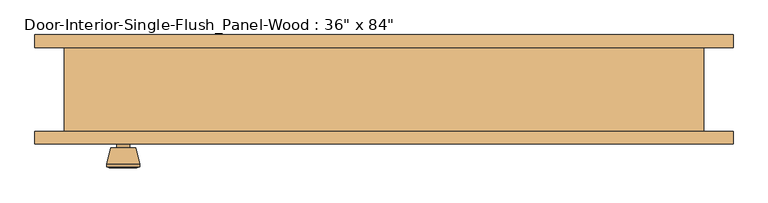
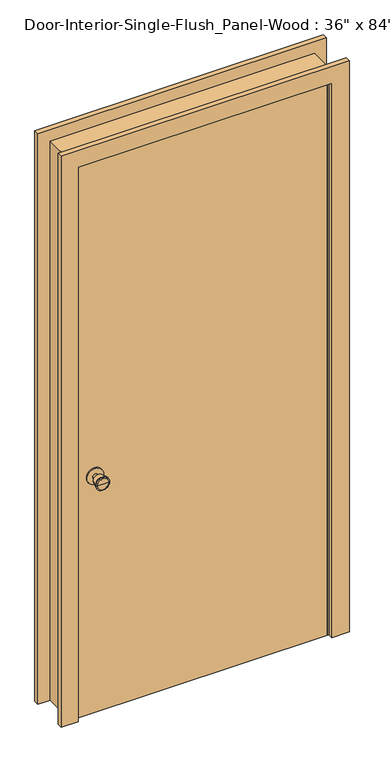
"""IFC4 building model written with IfcOpenShell, lengths in millimetres: door geometry."""

from ifc_helpers import new_model, si_unit, point, frame, frame_2d, origin, origin_with_axes, place, context, project, spatial, polyline, circle_curve, trimmed, segment, composite_curve, outline, extrude, faceted_brep, source, transform, mapped, element, save
from ifc_brep_helpers import plane_surface, cylinder_surface, revolved_surface, advanced_brep


def door_fdc9072e(model_context):
    return source(origin(), model_context, "Body", "SolidModel", [
        advanced_brep(
        [(-393.7, -19.4, 914.4), (-403.7, -19.4, 914.4), (-383.7, -19.4, 914.4), (-373.2241324, 29.6, 914.4), (-414.1758676, 29.6, 914.4), (-393.7, 29.6, 914.4), (-368.7, 27.7721319, 914.4), (-418.7, 27.7721319, 914.4), (-368.7, 24.3084537, 914.4), (-418.7, 24.3084537, 914.4), (-375.063764, -0.4, 914.4), (-412.336236, -0.4, 914.4), (-383.7, -0.4, 914.4), (-403.7, -0.4, 914.4)],
        [
            (0, 1),
            (1, 2, circle_curve(frame((-393.7, -19.4, 914.4), z_axis=(0.0, -1.0, 0.0), x_axis=(-1.0, 0.0, 0.0)), 10.0)),
            (2, 0),
            (2, 1, circle_curve(frame((-393.7, -19.4, 914.4), z_axis=(0.0, -1.0, 0.0), x_axis=(-1.0, 0.0, 0.0)), 10.0)),
            (3, 4, circle_curve(frame((-393.7, 29.6, 914.4), z_axis=(0.0, 1.0, 0.0), x_axis=(-1.0, 0.0, 0.0)), 20.4758676)),
            (4, 5),
            (5, 3),
            (4, 3, circle_curve(frame((-393.7, 29.6, 914.4), z_axis=(0.0, 1.0, 0.0), x_axis=(-1.0, 0.0, 0.0)), 20.4758676)),
            (6, 7, circle_curve(frame((-393.7, 27.7721319, 914.4), z_axis=(0.0, 1.0, 0.0), x_axis=(-1.0, 0.0, 0.0)), 25.0)),
            (7, 4),
            (3, 6),
            (7, 6, circle_curve(frame((-393.7, 27.7721319, 914.4), z_axis=(0.0, 1.0, 0.0), x_axis=(-1.0, 0.0, 0.0)), 25.0)),
            (8, 9, circle_curve(frame((-393.7, 24.3084537, 914.4), z_axis=(0.0, 1.0, 0.0), x_axis=(-1.0, 0.0, 0.0)), 25.0)),
            (9, 7),
            (6, 8),
            (9, 8, circle_curve(frame((-393.7, 24.3084537, 914.4), z_axis=(0.0, 1.0, 0.0), x_axis=(-1.0, 0.0, 0.0)), 25.0)),
            (10, 11, circle_curve(frame((-393.7, -0.4, 914.4), z_axis=(0.0, 1.0, 0.0), x_axis=(-1.0, 0.0, 0.0)), 18.636236)),
            (11, 9),
            (8, 10),
            (11, 10, circle_curve(frame((-393.7, -0.4, 914.4), z_axis=(0.0, 1.0, 0.0), x_axis=(-1.0, 0.0, 0.0)), 18.636236)),
            (12, 13, circle_curve(frame((-393.7, -0.4, 914.4), z_axis=(0.0, 1.0, 0.0), x_axis=(-1.0, 0.0, 0.0)), 10.0)),
            (13, 11),
            (10, 12),
            (13, 12, circle_curve(frame((-393.7, -0.4, 914.4), z_axis=(0.0, 1.0, 0.0), x_axis=(-1.0, 0.0, 0.0)), 10.0)),
            (1, 13),
            (12, 2),
        ],
        [
            plane_surface(frame((-393.7, -19.4, 914.4), z_axis=(0.0, -1.0, 0.0), x_axis=(-1.0, 0.0, 0.0))),
            plane_surface(frame((-393.7, 29.6, 914.4), z_axis=(0.0, 1.0, 0.0), x_axis=(-1.0, 0.0, 0.0))),
            revolved_surface(polyline([(-414.1758676, 29.6, 914.4), (-418.7, 27.7721319, 914.4)]), (-393.7, -19.4, 914.4), (0.0, -1.0, 0.0)),
            cylinder_surface(frame((-393.7, -19.4, 914.4), z_axis=(0.0, -1.0, 0.0), x_axis=(-1.0, 0.0, 0.0)), 25.0),
            revolved_surface(polyline([(-418.7, 24.3084537, 914.4), (-412.336236, -0.4, 914.4)]), (-393.7, -19.4, 914.4), (0.0, -1.0, 0.0)),
            plane_surface(frame((-393.7, -0.4, 914.4), z_axis=(0.0, -1.0, 0.0), x_axis=(-1.0, 0.0, 0.0))),
            cylinder_surface(frame((-393.7, -19.4, 914.4), z_axis=(0.0, -1.0, 0.0), x_axis=(-1.0, 0.0, 0.0)), 10.0),
        ],
        [
            (0, [[1, 2, 3]]),
            (0, [[-3, 4, -1]]),
            (1, [[5, 6, 7]]),
            (1, [[8, -7, -6]]),
            (2, [[9, 10, -5, 11]]),
            (2, [[12, -11, -8, -10]]),
            (3, [[13, 14, -9, 15]]),
            (3, [[16, -15, -12, -14]]),
            (4, [[17, 18, -13, 19]]),
            (4, [[20, -19, -16, -18]]),
            (5, [[21, 22, -17, 23]]),
            (5, [[24, -23, -20, -22]]),
            (6, [[-2, 25, -21, 26]]),
            (6, [[-4, -26, -24, -25]]),
        ],
    ),
        extrude(outline(composite_curve([segment(trimmed(circle_curve(frame_2d((914.4, -393.7)), 30.0), [point((914.4, -423.7))], [point((914.4, -363.7))], False, "CARTESIAN"), True, "CONTINUOUS"), segment(trimmed(circle_curve(frame_2d((914.4, -393.7)), 30.0), [point((914.4, -363.7))], [point((914.4, -423.7))], False, "CARTESIAN"), True, "CONTINUOUS")], self_intersect=False)), frame((0.0, -25.4, 0.0), z_axis=(0.0, 1.0, 0.0), x_axis=(0.0, 0.0, 1.0)), (0.0, 0.0, 1.0), 6.0),
        advanced_brep(
        [(-393.7, -66.325, 914.4), (-383.7, -66.325, 914.4), (-403.7, -66.325, 914.4), (-373.2241324, -115.325, 914.4), (-393.7, -115.325, 914.4), (-414.1758676, -115.325, 914.4), (-368.7, -113.4971319, 914.4), (-418.7, -113.4971319, 914.4), (-368.7, -110.0334537, 914.4), (-418.7, -110.0334537, 914.4), (-375.063764, -85.325, 914.4), (-412.336236, -85.325, 914.4), (-383.7, -85.325, 914.4), (-403.7, -85.325, 914.4)],
        [
            (0, 1),
            (1, 2, circle_curve(frame((-393.7, -66.325, 914.4), z_axis=(0.0, 1.0, 0.0), x_axis=(-1.0, 0.0, 0.0)), 10.0)),
            (2, 0),
            (2, 1, circle_curve(frame((-393.7, -66.325, 914.4), z_axis=(0.0, 1.0, 0.0), x_axis=(-1.0, 0.0, 0.0)), 10.0)),
            (3, 4),
            (4, 5),
            (5, 3, circle_curve(frame((-393.7, -115.325, 914.4), z_axis=(0.0, -1.0, 0.0), x_axis=(-1.0, 0.0, 0.0)), 20.4758676)),
            (3, 5, circle_curve(frame((-393.7, -115.325, 914.4), z_axis=(0.0, -1.0, 0.0), x_axis=(-1.0, 0.0, 0.0)), 20.4758676)),
            (6, 3),
            (5, 7),
            (7, 6, circle_curve(frame((-393.7, -113.4971319, 914.4), z_axis=(0.0, -1.0, 0.0), x_axis=(-1.0, 0.0, 0.0)), 25.0)),
            (6, 7, circle_curve(frame((-393.7, -113.4971319, 914.4), z_axis=(0.0, -1.0, 0.0), x_axis=(-1.0, 0.0, 0.0)), 25.0)),
            (8, 6),
            (7, 9),
            (9, 8, circle_curve(frame((-393.7, -110.0334537, 914.4), z_axis=(0.0, -1.0, 0.0), x_axis=(-1.0, 0.0, 0.0)), 25.0)),
            (8, 9, circle_curve(frame((-393.7, -110.0334537, 914.4), z_axis=(0.0, -1.0, 0.0), x_axis=(-1.0, 0.0, 0.0)), 25.0)),
            (10, 8),
            (9, 11),
            (11, 10, circle_curve(frame((-393.7, -85.325, 914.4), z_axis=(0.0, -1.0, 0.0), x_axis=(-1.0, 0.0, 0.0)), 18.636236)),
            (10, 11, circle_curve(frame((-393.7, -85.325, 914.4), z_axis=(0.0, -1.0, 0.0), x_axis=(-1.0, 0.0, 0.0)), 18.636236)),
            (12, 10),
            (11, 13),
            (13, 12, circle_curve(frame((-393.7, -85.325, 914.4), z_axis=(0.0, -1.0, 0.0), x_axis=(-1.0, 0.0, 0.0)), 10.0)),
            (12, 13, circle_curve(frame((-393.7, -85.325, 914.4), z_axis=(0.0, -1.0, 0.0), x_axis=(-1.0, 0.0, 0.0)), 10.0)),
            (1, 12),
            (13, 2),
        ],
        [
            plane_surface(frame((-393.7, -66.325, 914.4), z_axis=(0.0, 1.0, 0.0), x_axis=(-1.0, 0.0, 0.0))),
            plane_surface(frame((-393.7, -115.325, 914.4), z_axis=(0.0, -1.0, 0.0), x_axis=(-1.0, 0.0, 0.0))),
            revolved_surface(polyline([(-414.1758676, -115.325, 914.4), (-418.7, -113.4971319, 914.4)]), (-393.7, -66.325, 914.4), (0.0, 1.0, 0.0)),
            cylinder_surface(frame((-393.7, -66.325, 914.4), z_axis=(0.0, 1.0, 0.0), x_axis=(-1.0, 0.0, 0.0)), 25.0),
            revolved_surface(polyline([(-418.7, -110.0334537, 914.4), (-412.336236, -85.325, 914.4)]), (-393.7, -66.325, 914.4), (0.0, 1.0, 0.0)),
            plane_surface(frame((-393.7, -85.325, 914.4), z_axis=(0.0, 1.0, 0.0), x_axis=(-1.0, 0.0, 0.0))),
            cylinder_surface(frame((-393.7, -66.325, 914.4), z_axis=(0.0, 1.0, 0.0), x_axis=(-1.0, 0.0, 0.0)), 10.0),
        ],
        [
            (0, [[1, 2, 3]]),
            (0, [[-3, 4, -1]]),
            (1, [[5, 6, 7]]),
            (1, [[-6, -5, 8]]),
            (2, [[9, -7, 10, 11]]),
            (2, [[-10, -8, -9, 12]]),
            (3, [[13, -11, 14, 15]]),
            (3, [[-14, -12, -13, 16]]),
            (4, [[17, -15, 18, 19]]),
            (4, [[-18, -16, -17, 20]]),
            (5, [[21, -19, 22, 23]]),
            (5, [[-22, -20, -21, 24]]),
            (6, [[25, -23, 26, -2]]),
            (6, [[-26, -24, -25, -4]]),
        ],
    ),
        extrude(outline(composite_curve([segment(trimmed(circle_curve(frame_2d((914.4, -393.7)), 30.0), [point((914.4, -423.7))], [point((914.4, -363.7))], False, "CARTESIAN"), True, "CONTINUOUS"), segment(trimmed(circle_curve(frame_2d((914.4, -393.7)), 30.0), [point((914.4, -363.7))], [point((914.4, -423.7))], False, "CARTESIAN"), True, "CONTINUOUS")], self_intersect=False)), frame((0.0, -66.325, 0.0), z_axis=(0.0, 1.0, 0.0), x_axis=(0.0, 0.0, 1.0)), (0.0, 0.0, 1.0), 6.0),
        faceted_brep([(482.6, -60.325, 0.0), (457.2, -60.325, 0.0), (457.2, -25.4, 0.0), (444.5, -25.4, 0.0), (444.5, 9.525, 0.0), (457.2, 9.525, 0.0), (457.2, 66.675, 0.0), (482.6, 66.675, 0.0), (482.6, 66.675, 2159.0), (482.6, -60.325, 2159.0), (457.2, 66.675, 2133.6), (-457.2, 66.675, 2133.6), (-457.2, 66.675, 0.0), (-482.6, 66.675, 0.0), (-482.6, 66.675, 2159.0), (457.2, 9.525, 2133.6), (444.5, 9.525, 2120.9), (-444.5, 9.525, 2120.9), (-444.5, 9.525, 0.0), (-457.2, 9.525, 0.0), (-457.2, 9.525, 2133.6), (444.5, -25.4, 2120.9), (457.2, -25.4, 2133.6), (-457.2, -25.4, 2133.6), (-457.2, -25.4, 0.0), (-444.5, -25.4, 0.0), (-444.5, -25.4, 2120.9), (457.2, -60.325, 2133.6), (-482.6, -60.325, 2159.0), (-482.6, -60.325, 0.0), (-457.2, -60.325, 0.0), (-457.2, -60.325, 2133.6)], [[[0, 1, 2, 3, 4, 5, 6, 7]], [[7, 8, 9, 0]], [[6, 10, 11, 12, 13, 14, 8, 7]], [[5, 15, 10, 6]], [[4, 16, 17, 18, 19, 20, 15, 5]], [[3, 21, 16, 4]], [[2, 22, 23, 24, 25, 26, 21, 3]], [[1, 27, 22, 2]], [[0, 9, 28, 29, 30, 31, 27, 1]], [[8, 14, 28, 9]], [[15, 20, 11, 10]], [[21, 26, 17, 16]], [[27, 31, 23, 22]], [[29, 13, 12, 19, 18, 25, 24, 30]], [[14, 13, 29, 28]], [[20, 19, 12, 11]], [[26, 25, 18, 17]], [[31, 30, 24, 23]]]),
        extrude(outline(polyline([(457.2, -25.4), (457.2, -60.325), (-457.2, -60.325), (-457.2, -25.4), (457.2, -25.4)])), origin_with_axes(), (0.0, 0.0, 1.0), 2133.6),
        extrude(outline(polyline([(0.0, 527.05), (2203.45, 527.05), (2203.45, -527.05), (0.0, -527.05), (0.0, -463.55), (2139.95, -463.55), (2139.95, 463.55), (0.0, 463.55), (0.0, 527.05)])), frame((0.0, -79.375, 0.0), z_axis=(0.0, 1.0, 0.0), x_axis=(0.0, 0.0, 1.0)), (0.0, 0.0, 1.0), 19.05),
        extrude(outline(polyline([(0.0, 527.05), (2203.45, 527.05), (2203.45, -527.05), (0.0, -527.05), (0.0, -463.55), (2139.95, -463.55), (2139.95, 463.55), (0.0, 463.55), (0.0, 527.05)])), frame((0.0, 66.675, 0.0), z_axis=(0.0, 1.0, 0.0), x_axis=(0.0, 0.0, 1.0)), (0.0, 0.0, 1.0), 19.05),
    ])


if __name__ == "__main__":
    model = new_model("IFC4")
    model_context = context("Model", 3, world=origin())
    ifc_project = project(units=[si_unit("LENGTHUNIT", "METRE", prefix="MILLI")], contexts=[model_context])
    site = spatial("IfcSite", under=ifc_project)
    building = spatial("IfcBuilding", under=site)
    placement = place(None, origin())
    door_shape = door_fdc9072e(model_context)
    element("IfcDoor", 1, ObjectType="Door-Interior-Single-Flush_Panel-Wood : 36\" x 84\"", at=placement, inside=building, context=model_context, shape_type="MappedRepresentation", body=[
        mapped(door_shape, transform((0.0, 0.0, 0.0), x_axis=(1.0, 0.0, 0.0), y_axis=(0.0, 1.0, 0.0), z_axis=(0.0, 0.0, 1.0))),
    ])
    save(model, "model.ifc")

# Revit data of these elements
# Type "Door-Interior-Single-Flush_Panel-Wood : 36\" x 84\""
#   Type Mark = "8"
#   Assembly Code = "C1020300"
#   Analytic Construction = "Wooden"
#   Thickness = 0' - 1 3/8"
#   Thermal Resistance (R) = 2.5876 (h·ft²·°F)/BTU
#   Swing Angle [instance default] = 90.00°
#   Rough Width = 3' - 2"
#   Rough Height = 7' - 1"
#   Height = 7' - 0"
#   Width = 3' - 0"
#   Heat Transfer Coefficient (U) = 0.3865 BTU/(h·ft²·°F)
#   Trim Material = Cherry
#   Panel Material = Cherry
#   Frame Material = Cherry
#   Door Handle Material = Aluminum
#   Visual Light Transmittance = 0
#   Solar Heat Gain Coefficient = 0
#   Wall Closure = (empty or 0)
#   Function = (empty or 0)
# Element 1 (IfcDoor, "Door-Interior-Single-Flush_Panel-Wood : 36\" x 84\"")
#   Materials on its faces: "Cherry", "Aluminum"
# Materials
#   "Cherry": class "Wood", colour RGB 226 177 128, transparency 0, Description = "Prunus Serotina", Cost = 0
#   "Aluminum": class "Metal", colour RGB 247 247 247, transparency 0, Description = "Aluminum 6061", Cost = 0
